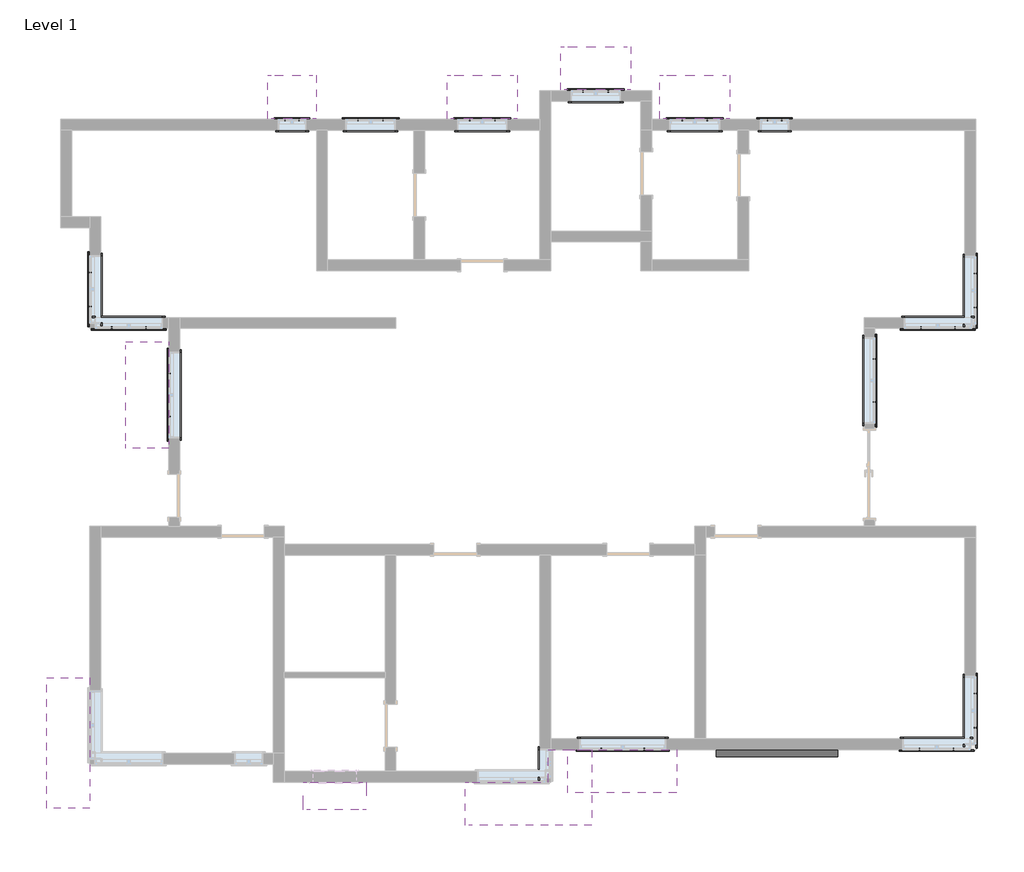
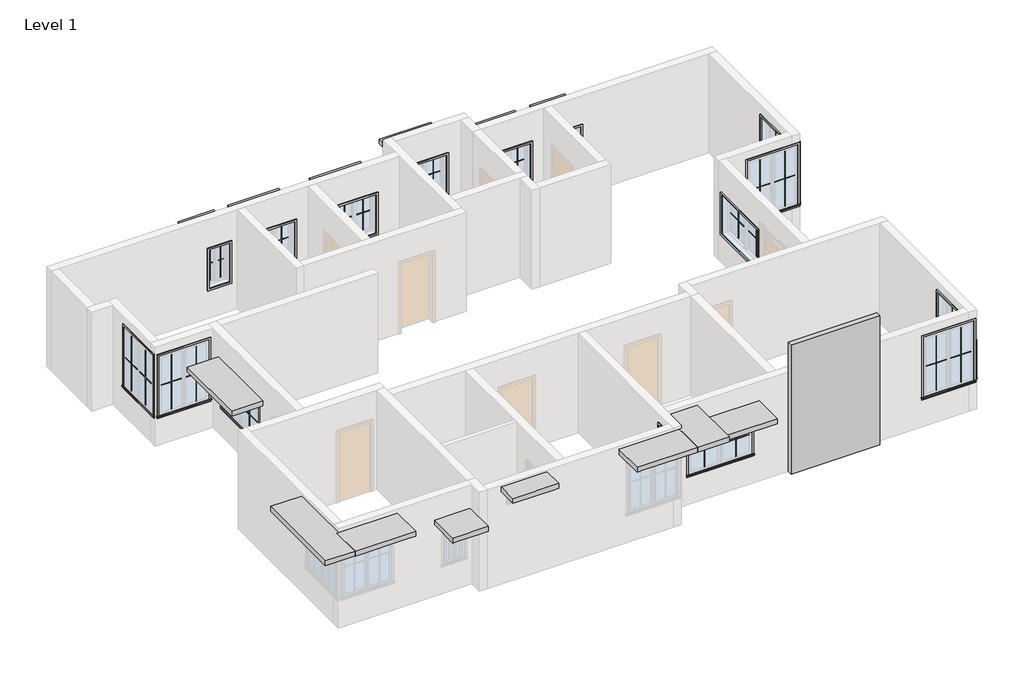
# One storey, part 3 of 3: 71 proxies.
"""IFC4 building model written with IfcOpenShell, lengths in millimetres."""

from ifc_helpers import new_model, si_unit, origin, place, context, project, spatial, transform, mapped, element, save
from components import generic_models_1_generic_models_1_0485f0a6, generic_models_13_generic_models_13_60817c59, generic_models_2_generic_models_2_5dfb3e49, generic_models_3_generic_models_3_1965cac1, generic_models_4_generic_models_4_668f170e, generic_models_5_generic_models_5_4455ebe8, generic_models_6_generic_models_6_772fa5ba, generic_models_7_generic_models_7_55042171, generic_models_8_generic_models_8_7ecb40ae, generic_models_9_generic_models_9_114c8f56, muntin_pattern_2x2_muntin_pattern_2x2_ddac5204, muntin_pattern_2x2_muntin_pattern_2x2_784a3213, muntin_pattern_2x2_muntin_pattern_2x2_dc2504c2, muntin_pattern_2x2_muntin_pattern_2x2_0aa094e9, muntin_pattern_2x2_muntin_pattern_2x2_63e5058f, muntin_pattern_2x2_muntin_pattern_2x2_529c3de1, muntin_pattern_2x2_muntin_pattern_2x2_bff912c5, muntin_pattern_2x2_muntin_pattern_2x2_c2194282, trim_window_exterior_flat_with_sill_35723329, trim_window_exterior_flat_with_sill_02d88a07, trim_window_exterior_flat_with_sill_245f2bb1, trim_window_exterior_flat_with_sill_e04b3088, trim_window_interior_flat_picture_frame_e16bff95, trim_window_interior_flat_picture_frame_03e64d7c, trim_window_interior_flat_picture_frame_2b4ba637, trim_window_interior_flat_picture_frame_2a7685fe, trim_window_interior_flat_picture_frame_6ac783dc

model = new_model("IFC4")

# Units and contexts
model_context = context("Model", 3, world=origin())
ifc_project = project(units=[si_unit("LENGTHUNIT", "METRE", prefix="MILLI")], contexts=[model_context])

# Site, building, storey
site = spatial("IfcSite", under=ifc_project)
building = spatial("IfcBuilding", under=site)
storey = spatial("IfcBuildingStorey", under=building, Name="Level 1", Elevation=0.0)

# Proxies
placement = place(None, origin())
generic_models_1_generic_models_1_shape = generic_models_1_generic_models_1_0485f0a6(model_context)
element("IfcBuildingElementProxy", 1, Name="Generic Models 1 : Generic Models 1", ObjectType="Generic Models 1 : Generic Models 1", at=placement, inside=storey, context=model_context, shape_type="MappedRepresentation", body=[
    mapped(generic_models_1_generic_models_1_shape, transform((0.0, 0.0, 0.0), x_axis=(1.0, 0.0, 0.0), y_axis=(0.0, 1.0, 0.0), z_axis=(0.0, 0.0, 1.0))),
])
generic_models_13_generic_models_13_shape = generic_models_13_generic_models_13_60817c59(model_context)
element("IfcBuildingElementProxy", 2, Name="Generic Models 13 : Generic Models 13", ObjectType="Generic Models 13 : Generic Models 13", at=placement, inside=storey, context=model_context, shape_type="MappedRepresentation", body=[
    mapped(generic_models_13_generic_models_13_shape, transform((0.0, 0.0, 0.0), x_axis=(1.0, 0.0, 0.0), y_axis=(0.0, 1.0, 0.0), z_axis=(0.0, 0.0, 1.0))),
])
generic_models_2_generic_models_2_shape = generic_models_2_generic_models_2_5dfb3e49(model_context)
element("IfcBuildingElementProxy", 3, Name="Generic Models 2 : Generic Models 2", ObjectType="Generic Models 2 : Generic Models 2", at=placement, inside=storey, context=model_context, shape_type="MappedRepresentation", body=[
    mapped(generic_models_2_generic_models_2_shape, transform((0.0, 0.0, 0.0), x_axis=(1.0, 0.0, 0.0), y_axis=(0.0, 1.0, 0.0), z_axis=(0.0, 0.0, 1.0))),
])
generic_models_3_generic_models_3_shape = generic_models_3_generic_models_3_1965cac1(model_context)
element("IfcBuildingElementProxy", 4, Name="Generic Models 3 : Generic Models 3", ObjectType="Generic Models 3 : Generic Models 3", at=placement, inside=storey, context=model_context, shape_type="MappedRepresentation", body=[
    mapped(generic_models_3_generic_models_3_shape, transform((-51.3527819, 0.0, 0.0272468), x_axis=(1.0, 0.0, 0.0), y_axis=(0.0, 1.0, 0.0), z_axis=(0.0, 0.0, 1.0))),
])
generic_models_4_generic_models_4_shape = generic_models_4_generic_models_4_668f170e(model_context)
element("IfcBuildingElementProxy", 5, Name="Generic Models 4 : Generic Models 4", ObjectType="Generic Models 4 : Generic Models 4", at=placement, inside=storey, context=model_context, shape_type="MappedRepresentation", body=[
    mapped(generic_models_4_generic_models_4_shape, transform((0.0, 0.0, 0.0), x_axis=(1.0, 0.0, 0.0), y_axis=(0.0, 1.0, 0.0), z_axis=(0.0, 0.0, 1.0))),
])
generic_models_5_generic_models_5_shape = generic_models_5_generic_models_5_4455ebe8(model_context)
element("IfcBuildingElementProxy", 6, Name="Generic Models 5 : Generic Models 5", ObjectType="Generic Models 5 : Generic Models 5", at=placement, inside=storey, context=model_context, shape_type="MappedRepresentation", body=[
    mapped(generic_models_5_generic_models_5_shape, transform((0.0, 0.0, 0.0), x_axis=(1.0, 0.0, 0.0), y_axis=(0.0, 1.0, 0.0), z_axis=(0.0, 0.0, 1.0))),
])
generic_models_6_generic_models_6_shape = generic_models_6_generic_models_6_772fa5ba(model_context)
element("IfcBuildingElementProxy", 7, Name="Generic Models 6 : Generic Models 6", ObjectType="Generic Models 6 : Generic Models 6", at=placement, inside=storey, context=model_context, shape_type="MappedRepresentation", body=[
    mapped(generic_models_6_generic_models_6_shape, transform((0.0, 0.0, 0.0), x_axis=(1.0, 0.0, 0.0), y_axis=(0.0, 1.0, 0.0), z_axis=(0.0, 0.0, 1.0))),
])
generic_models_7_generic_models_7_shape = generic_models_7_generic_models_7_55042171(model_context)
element("IfcBuildingElementProxy", 8, Name="Generic Models 7 : Generic Models 7", ObjectType="Generic Models 7 : Generic Models 7", at=placement, inside=storey, context=model_context, shape_type="MappedRepresentation", body=[
    mapped(generic_models_7_generic_models_7_shape, transform((0.0, 0.0, 0.0), x_axis=(1.0, 0.0, 0.0), y_axis=(0.0, 1.0, 0.0), z_axis=(0.0, 0.0, 1.0))),
])
generic_models_8_generic_models_8_shape = generic_models_8_generic_models_8_7ecb40ae(model_context)
element("IfcBuildingElementProxy", 9, Name="Generic Models 8 : Generic Models 8", ObjectType="Generic Models 8 : Generic Models 8", at=placement, inside=storey, context=model_context, shape_type="MappedRepresentation", body=[
    mapped(generic_models_8_generic_models_8_shape, transform((0.0, 0.0, 0.0), x_axis=(1.0, 0.0, 0.0), y_axis=(0.0, 1.0, 0.0), z_axis=(0.0, 0.0, 1.0))),
])
generic_models_9_generic_models_9_shape = generic_models_9_generic_models_9_114c8f56(model_context)
element("IfcBuildingElementProxy", 10, Name="Generic Models 9 : Generic Models 9", ObjectType="Generic Models 9 : Generic Models 9", at=placement, inside=storey, context=model_context, shape_type="MappedRepresentation", body=[
    mapped(generic_models_9_generic_models_9_shape, transform((0.0, 0.0, 0.0), x_axis=(1.0, 0.0, 0.0), y_axis=(0.0, 1.0, 0.0), z_axis=(0.0, 0.0, 1.0))),
])
muntin_pattern_2x2_muntin_pattern_2x2_shape = muntin_pattern_2x2_muntin_pattern_2x2_ddac5204(model_context)
element("IfcBuildingElementProxy", 11, Name="Muntin Pattern_2x2 : Muntin Pattern_2x2", ObjectType="Muntin Pattern_2x2 : Muntin Pattern_2x2", at=placement, inside=storey, context=model_context, shape_type="MappedRepresentation", body=[
    mapped(muntin_pattern_2x2_muntin_pattern_2x2_shape, transform((-27733.7270004, 19654.2006148, 984.25), x_axis=(1.0, 0.0, 0.0), y_axis=(0.0, 1.0, 0.0), z_axis=(0.0, 0.0, 1.0))),
])
element("IfcBuildingElementProxy", 12, Name="Muntin Pattern_2x2 : Muntin Pattern_2x2", ObjectType="Muntin Pattern_2x2 : Muntin Pattern_2x2", at=placement, inside=storey, context=model_context, shape_type="MappedRepresentation", body=[
    mapped(muntin_pattern_2x2_muntin_pattern_2x2_shape, transform((-37944.5270004, 19654.2006148, 984.25), x_axis=(1.0, 0.0, 0.0), y_axis=(0.0, 1.0, 0.0), z_axis=(0.0, 0.0, 1.0))),
])
muntin_pattern_2x2_muntin_pattern_2x2_2_shape = muntin_pattern_2x2_muntin_pattern_2x2_784a3213(model_context)
element("IfcBuildingElementProxy", 13, Name="Muntin Pattern_2x2 : Muntin Pattern_2x2", ObjectType="Muntin Pattern_2x2 : Muntin Pattern_2x2", at=placement, inside=storey, context=model_context, shape_type="MappedRepresentation", body=[
    mapped(muntin_pattern_2x2_muntin_pattern_2x2_2_shape, transform((-27432.1020004, 19654.2006148, 984.25), x_axis=(-1.0, 0.0, 0.0), y_axis=(0.0, -1.0, 0.0), z_axis=(0.0, 0.0, 1.0))),
])
element("IfcBuildingElementProxy", 14, Name="Muntin Pattern_2x2 : Muntin Pattern_2x2", ObjectType="Muntin Pattern_2x2 : Muntin Pattern_2x2", at=placement, inside=storey, context=model_context, shape_type="MappedRepresentation", body=[
    mapped(muntin_pattern_2x2_muntin_pattern_2x2_2_shape, transform((-37642.9020004, 19654.2006148, 984.25), x_axis=(-1.0, 0.0, 0.0), y_axis=(0.0, -1.0, 0.0), z_axis=(0.0, 0.0, 1.0))),
])
muntin_pattern_2x2_muntin_pattern_2x2_3_shape = muntin_pattern_2x2_muntin_pattern_2x2_dc2504c2(model_context)
element("IfcBuildingElementProxy", 15, Name="Muntin Pattern_2x2 : Muntin Pattern_2x2", ObjectType="Muntin Pattern_2x2 : Muntin Pattern_2x2", at=placement, inside=storey, context=model_context, shape_type="MappedRepresentation", body=[
    mapped(muntin_pattern_2x2_muntin_pattern_2x2_3_shape, transform((-30340.4020004, 6338.2506148, 984.25), x_axis=(-1.0, 0.0, 0.0), y_axis=(0.0, -1.0, 0.0), z_axis=(0.0, 0.0, 1.0))),
])
element("IfcBuildingElementProxy", 16, Name="Muntin Pattern_2x2 : Muntin Pattern_2x2", ObjectType="Muntin Pattern_2x2 : Muntin Pattern_2x2", at=placement, inside=storey, context=model_context, shape_type="MappedRepresentation", body=[
    mapped(muntin_pattern_2x2_muntin_pattern_2x2_3_shape, transform((-25471.5395004, 14594.8381148, 984.25), x_axis=(0.0, -1.0, 0.0), y_axis=(1.0, 0.0, 0.0), z_axis=(0.0, 0.0, 1.0))),
])
element("IfcBuildingElementProxy", 17, Name="Muntin Pattern_2x2 : Muntin Pattern_2x2", ObjectType="Muntin Pattern_2x2 : Muntin Pattern_2x2", at=placement, inside=storey, context=model_context, shape_type="MappedRepresentation", body=[
    mapped(muntin_pattern_2x2_muntin_pattern_2x2_3_shape, transform((-40387.6895004, 13378.8131148, 984.25), x_axis=(0.0, 1.0, 0.0), y_axis=(-1.0, 0.0, 0.0), z_axis=(0.0, 0.0, 1.0))),
])
muntin_pattern_2x2_muntin_pattern_2x2_4_shape = muntin_pattern_2x2_muntin_pattern_2x2_0aa094e9(model_context)
element("IfcBuildingElementProxy", 18, Name="Muntin Pattern_2x2 : Muntin Pattern_2x2", ObjectType="Muntin Pattern_2x2 : Muntin Pattern_2x2", at=placement, inside=storey, context=model_context, shape_type="MappedRepresentation", body=[
    mapped(muntin_pattern_2x2_muntin_pattern_2x2_4_shape, transform((-31251.6270004, 6338.2506148, 984.25), x_axis=(1.0, 0.0, 0.0), y_axis=(0.0, 1.0, 0.0), z_axis=(0.0, 0.0, 1.0))),
])
element("IfcBuildingElementProxy", 19, Name="Muntin Pattern_2x2 : Muntin Pattern_2x2", ObjectType="Muntin Pattern_2x2 : Muntin Pattern_2x2", at=placement, inside=storey, context=model_context, shape_type="MappedRepresentation", body=[
    mapped(muntin_pattern_2x2_muntin_pattern_2x2_4_shape, transform((-25471.5395004, 13683.6131148, 984.25), x_axis=(0.0, 1.0, 0.0), y_axis=(-1.0, 0.0, 0.0), z_axis=(0.0, 0.0, 1.0))),
])
element("IfcBuildingElementProxy", 20, Name="Muntin Pattern_2x2 : Muntin Pattern_2x2", ObjectType="Muntin Pattern_2x2 : Muntin Pattern_2x2", at=placement, inside=storey, context=model_context, shape_type="MappedRepresentation", body=[
    mapped(muntin_pattern_2x2_muntin_pattern_2x2_4_shape, transform((-40387.6895004, 14290.0381148, 984.25), x_axis=(0.0, -1.0, 0.0), y_axis=(1.0, 0.0, 0.0), z_axis=(0.0, 0.0, 1.0))),
])
muntin_pattern_2x2_muntin_pattern_2x2_5_shape = muntin_pattern_2x2_muntin_pattern_2x2_63e5058f(model_context)
element("IfcBuildingElementProxy", 21, Name="Muntin Pattern_2x2 : Muntin Pattern_2x2", ObjectType="Muntin Pattern_2x2 : Muntin Pattern_2x2", at=placement, inside=storey, context=model_context, shape_type="MappedRepresentation", body=[
    mapped(muntin_pattern_2x2_muntin_pattern_2x2_5_shape, transform((-36395.1270004, 19654.2006148, 984.25), x_axis=(1.0, 0.0, 0.0), y_axis=(0.0, 1.0, 0.0), z_axis=(0.0, 0.0, 1.0))),
])
element("IfcBuildingElementProxy", 22, Name="Muntin Pattern_2x2 : Muntin Pattern_2x2", ObjectType="Muntin Pattern_2x2 : Muntin Pattern_2x2", at=placement, inside=storey, context=model_context, shape_type="MappedRepresentation", body=[
    mapped(muntin_pattern_2x2_muntin_pattern_2x2_5_shape, transform((-34032.9270004, 19654.2006148, 984.25), x_axis=(1.0, 0.0, 0.0), y_axis=(0.0, 1.0, 0.0), z_axis=(0.0, 0.0, 1.0))),
])
element("IfcBuildingElementProxy", 23, Name="Muntin Pattern_2x2 : Muntin Pattern_2x2", ObjectType="Muntin Pattern_2x2 : Muntin Pattern_2x2", at=placement, inside=storey, context=model_context, shape_type="MappedRepresentation", body=[
    mapped(muntin_pattern_2x2_muntin_pattern_2x2_5_shape, transform((-31632.6270004, 20263.8006148, 984.25), x_axis=(1.0, 0.0, 0.0), y_axis=(0.0, 1.0, 0.0), z_axis=(0.0, 0.0, 1.0))),
])
element("IfcBuildingElementProxy", 24, Name="Muntin Pattern_2x2 : Muntin Pattern_2x2", ObjectType="Muntin Pattern_2x2 : Muntin Pattern_2x2", at=placement, inside=storey, context=model_context, shape_type="MappedRepresentation", body=[
    mapped(muntin_pattern_2x2_muntin_pattern_2x2_5_shape, transform((-29537.1270004, 19654.2006148, 984.25), x_axis=(1.0, 0.0, 0.0), y_axis=(0.0, 1.0, 0.0), z_axis=(0.0, 0.0, 1.0))),
])
muntin_pattern_2x2_muntin_pattern_2x2_6_shape = muntin_pattern_2x2_muntin_pattern_2x2_529c3de1(model_context)
element("IfcBuildingElementProxy", 25, Name="Muntin Pattern_2x2 : Muntin Pattern_2x2", ObjectType="Muntin Pattern_2x2 : Muntin Pattern_2x2", at=placement, inside=storey, context=model_context, shape_type="MappedRepresentation", body=[
    mapped(muntin_pattern_2x2_muntin_pattern_2x2_6_shape, transform((-35864.9020004, 19654.2006148, 984.25), x_axis=(-1.0, 0.0, 0.0), y_axis=(0.0, -1.0, 0.0), z_axis=(0.0, 0.0, 1.0))),
])
element("IfcBuildingElementProxy", 26, Name="Muntin Pattern_2x2 : Muntin Pattern_2x2", ObjectType="Muntin Pattern_2x2 : Muntin Pattern_2x2", at=placement, inside=storey, context=model_context, shape_type="MappedRepresentation", body=[
    mapped(muntin_pattern_2x2_muntin_pattern_2x2_6_shape, transform((-33502.7020004, 19654.2006148, 984.25), x_axis=(-1.0, 0.0, 0.0), y_axis=(0.0, -1.0, 0.0), z_axis=(0.0, 0.0, 1.0))),
])
element("IfcBuildingElementProxy", 27, Name="Muntin Pattern_2x2 : Muntin Pattern_2x2", ObjectType="Muntin Pattern_2x2 : Muntin Pattern_2x2", at=placement, inside=storey, context=model_context, shape_type="MappedRepresentation", body=[
    mapped(muntin_pattern_2x2_muntin_pattern_2x2_6_shape, transform((-31102.4020004, 20263.8006148, 984.25), x_axis=(-1.0, 0.0, 0.0), y_axis=(0.0, -1.0, 0.0), z_axis=(0.0, 0.0, 1.0))),
])
element("IfcBuildingElementProxy", 28, Name="Muntin Pattern_2x2 : Muntin Pattern_2x2", ObjectType="Muntin Pattern_2x2 : Muntin Pattern_2x2", at=placement, inside=storey, context=model_context, shape_type="MappedRepresentation", body=[
    mapped(muntin_pattern_2x2_muntin_pattern_2x2_6_shape, transform((-29006.9020004, 19654.2006148, 984.25), x_axis=(-1.0, 0.0, 0.0), y_axis=(0.0, -1.0, 0.0), z_axis=(0.0, 0.0, 1.0))),
])
muntin_pattern_2x2_muntin_pattern_2x2_7_shape = muntin_pattern_2x2_muntin_pattern_2x2_bff912c5(model_context)
element("IfcBuildingElementProxy", 29, Name="Muntin Pattern_2x2 : Muntin Pattern_2x2", ObjectType="Muntin Pattern_2x2 : Muntin Pattern_2x2", at=placement, inside=storey, context=model_context, shape_type="MappedRepresentation", body=[
    mapped(muntin_pattern_2x2_muntin_pattern_2x2_7_shape, transform((-23793.5520004, 6338.2506148, 984.25), x_axis=(-1.0, 0.0, 0.0), y_axis=(0.0, -1.0, 0.0), z_axis=(0.0, 0.0, 1.0))),
])
element("IfcBuildingElementProxy", 30, Name="Muntin Pattern_2x2 : Muntin Pattern_2x2", ObjectType="Muntin Pattern_2x2 : Muntin Pattern_2x2", at=placement, inside=storey, context=model_context, shape_type="MappedRepresentation", body=[
    mapped(muntin_pattern_2x2_muntin_pattern_2x2_7_shape, transform((-23337.9395004, 7514.5881148, 984.25), x_axis=(0.0, -1.0, 0.0), y_axis=(1.0, 0.0, 0.0), z_axis=(0.0, 0.0, 1.0))),
])
element("IfcBuildingElementProxy", 31, Name="Muntin Pattern_2x2 : Muntin Pattern_2x2", ObjectType="Muntin Pattern_2x2 : Muntin Pattern_2x2", at=placement, inside=storey, context=model_context, shape_type="MappedRepresentation", body=[
    mapped(muntin_pattern_2x2_muntin_pattern_2x2_7_shape, transform((-23768.1520004, 15253.6506148, 984.25), x_axis=(-1.0, 0.0, 0.0), y_axis=(0.0, -1.0, 0.0), z_axis=(0.0, 0.0, 1.0))),
])
element("IfcBuildingElementProxy", 32, Name="Muntin Pattern_2x2 : Muntin Pattern_2x2", ObjectType="Muntin Pattern_2x2 : Muntin Pattern_2x2", at=placement, inside=storey, context=model_context, shape_type="MappedRepresentation", body=[
    mapped(muntin_pattern_2x2_muntin_pattern_2x2_7_shape, transform((-23337.9395004, 16404.5881148, 984.25), x_axis=(0.0, -1.0, 0.0), y_axis=(1.0, 0.0, 0.0), z_axis=(0.0, 0.0, 1.0))),
])
element("IfcBuildingElementProxy", 33, Name="Muntin Pattern_2x2 : Muntin Pattern_2x2", ObjectType="Muntin Pattern_2x2 : Muntin Pattern_2x2", at=placement, inside=storey, context=model_context, shape_type="MappedRepresentation", body=[
    mapped(muntin_pattern_2x2_muntin_pattern_2x2_7_shape, transform((-40887.7520004, 15253.6506148, 984.25), x_axis=(-1.0, 0.0, 0.0), y_axis=(0.0, -1.0, 0.0), z_axis=(0.0, 0.0, 1.0))),
])
element("IfcBuildingElementProxy", 34, Name="Muntin Pattern_2x2 : Muntin Pattern_2x2", ObjectType="Muntin Pattern_2x2 : Muntin Pattern_2x2", at=placement, inside=storey, context=model_context, shape_type="MappedRepresentation", body=[
    mapped(muntin_pattern_2x2_muntin_pattern_2x2_7_shape, transform((-42064.0895004, 15709.2631148, 984.25), x_axis=(0.0, 1.0, 0.0), y_axis=(-1.0, 0.0, 0.0), z_axis=(0.0, 0.0, 1.0))),
])
muntin_pattern_2x2_muntin_pattern_2x2_8_shape = muntin_pattern_2x2_muntin_pattern_2x2_c2194282(model_context)
element("IfcBuildingElementProxy", 35, Name="Muntin Pattern_2x2 : Muntin Pattern_2x2", ObjectType="Muntin Pattern_2x2 : Muntin Pattern_2x2", at=placement, inside=storey, context=model_context, shape_type="MappedRepresentation", body=[
    mapped(muntin_pattern_2x2_muntin_pattern_2x2_8_shape, transform((-24514.2770004, 6338.2506148, 984.25), x_axis=(1.0, 0.0, 0.0), y_axis=(0.0, 1.0, 0.0), z_axis=(0.0, 0.0, 1.0))),
])
element("IfcBuildingElementProxy", 36, Name="Muntin Pattern_2x2 : Muntin Pattern_2x2", ObjectType="Muntin Pattern_2x2 : Muntin Pattern_2x2", at=placement, inside=storey, context=model_context, shape_type="MappedRepresentation", body=[
    mapped(muntin_pattern_2x2_muntin_pattern_2x2_8_shape, transform((-23337.9395004, 6793.8631148, 984.25), x_axis=(0.0, 1.0, 0.0), y_axis=(-1.0, 0.0, 0.0), z_axis=(0.0, 0.0, 1.0))),
])
element("IfcBuildingElementProxy", 37, Name="Muntin Pattern_2x2 : Muntin Pattern_2x2", ObjectType="Muntin Pattern_2x2 : Muntin Pattern_2x2", at=placement, inside=storey, context=model_context, shape_type="MappedRepresentation", body=[
    mapped(muntin_pattern_2x2_muntin_pattern_2x2_8_shape, transform((-24488.8770004, 15253.6506148, 984.25), x_axis=(1.0, 0.0, 0.0), y_axis=(0.0, 1.0, 0.0), z_axis=(0.0, 0.0, 1.0))),
])
element("IfcBuildingElementProxy", 38, Name="Muntin Pattern_2x2 : Muntin Pattern_2x2", ObjectType="Muntin Pattern_2x2 : Muntin Pattern_2x2", at=placement, inside=storey, context=model_context, shape_type="MappedRepresentation", body=[
    mapped(muntin_pattern_2x2_muntin_pattern_2x2_8_shape, transform((-23337.9395004, 15683.8631148, 984.25), x_axis=(0.0, 1.0, 0.0), y_axis=(-1.0, 0.0, 0.0), z_axis=(0.0, 0.0, 1.0))),
])
element("IfcBuildingElementProxy", 39, Name="Muntin Pattern_2x2 : Muntin Pattern_2x2", ObjectType="Muntin Pattern_2x2 : Muntin Pattern_2x2", at=placement, inside=storey, context=model_context, shape_type="MappedRepresentation", body=[
    mapped(muntin_pattern_2x2_muntin_pattern_2x2_8_shape, transform((-41608.4770004, 15253.6506148, 984.25), x_axis=(1.0, 0.0, 0.0), y_axis=(0.0, 1.0, 0.0), z_axis=(0.0, 0.0, 1.0))),
])
element("IfcBuildingElementProxy", 40, Name="Muntin Pattern_2x2 : Muntin Pattern_2x2", ObjectType="Muntin Pattern_2x2 : Muntin Pattern_2x2", at=placement, inside=storey, context=model_context, shape_type="MappedRepresentation", body=[
    mapped(muntin_pattern_2x2_muntin_pattern_2x2_8_shape, transform((-42064.0895004, 16429.9881148, 984.25), x_axis=(0.0, -1.0, 0.0), y_axis=(1.0, 0.0, 0.0), z_axis=(0.0, 0.0, 1.0))),
])
trim_window_exterior_flat_with_sill_shape = trim_window_exterior_flat_with_sill_35723329(model_context)
element("IfcBuildingElementProxy", 41, Name="Trim-Window-Exterior-Flat : with Sill", ObjectType="Trim-Window-Exterior-Flat : with Sill", at=placement, inside=storey, context=model_context, shape_type="MappedRepresentation", body=[
    mapped(trim_window_exterior_flat_with_sill_shape, transform((-27582.9145004, 19663.7256148, 2133.6), x_axis=(-1.0, 0.0, 0.0), y_axis=(0.0, 0.0, 1.0), z_axis=(0.0, 1.0, 0.0))),
])
element("IfcBuildingElementProxy", 42, Name="Trim-Window-Exterior-Flat : with Sill", ObjectType="Trim-Window-Exterior-Flat : with Sill", at=placement, inside=storey, context=model_context, shape_type="MappedRepresentation", body=[
    mapped(trim_window_exterior_flat_with_sill_shape, transform((-37793.7145004, 19663.7256148, 2133.6), x_axis=(-1.0, 0.0, 0.0), y_axis=(0.0, 0.0, 1.0), z_axis=(0.0, 1.0, 0.0))),
])
trim_window_exterior_flat_with_sill_2_shape = trim_window_exterior_flat_with_sill_02d88a07(model_context)
element("IfcBuildingElementProxy", 43, Name="Trim-Window-Exterior-Flat : with Sill", ObjectType="Trim-Window-Exterior-Flat : with Sill", at=placement, inside=storey, context=model_context, shape_type="MappedRepresentation", body=[
    mapped(trim_window_exterior_flat_with_sill_2_shape, transform((-30796.0145004, 6328.7256148, 2133.6), x_axis=(1.0, 0.0, 0.0), y_axis=(0.0, 0.0, 1.0), z_axis=(0.0, -1.0, 0.0))),
])
element("IfcBuildingElementProxy", 44, Name="Trim-Window-Exterior-Flat : with Sill", ObjectType="Trim-Window-Exterior-Flat : with Sill", at=placement, inside=storey, context=model_context, shape_type="MappedRepresentation", body=[
    mapped(trim_window_exterior_flat_with_sill_2_shape, transform((-25462.0145004, 14139.2256148, 2133.6), x_axis=(0.0, 1.0, 0.0), y_axis=(0.0, 0.0, 1.0), z_axis=(1.0, 0.0, 0.0))),
])
element("IfcBuildingElementProxy", 45, Name="Trim-Window-Exterior-Flat : with Sill", ObjectType="Trim-Window-Exterior-Flat : with Sill", at=placement, inside=storey, context=model_context, shape_type="MappedRepresentation", body=[
    mapped(trim_window_exterior_flat_with_sill_2_shape, transform((-40397.2145004, 13834.4256148, 2133.6), x_axis=(0.0, -1.0, 0.0), y_axis=(0.0, 0.0, 1.0), z_axis=(-1.0, 0.0, 0.0))),
])
trim_window_exterior_flat_with_sill_3_shape = trim_window_exterior_flat_with_sill_245f2bb1(model_context)
element("IfcBuildingElementProxy", 46, Name="Trim-Window-Exterior-Flat : with Sill", ObjectType="Trim-Window-Exterior-Flat : with Sill", at=placement, inside=storey, context=model_context, shape_type="MappedRepresentation", body=[
    mapped(trim_window_exterior_flat_with_sill_3_shape, transform((-36130.0145004, 19663.7256148, 2133.6), x_axis=(-1.0, 0.0, 0.0), y_axis=(0.0, 0.0, 1.0), z_axis=(0.0, 1.0, 0.0))),
])
element("IfcBuildingElementProxy", 47, Name="Trim-Window-Exterior-Flat : with Sill", ObjectType="Trim-Window-Exterior-Flat : with Sill", at=placement, inside=storey, context=model_context, shape_type="MappedRepresentation", body=[
    mapped(trim_window_exterior_flat_with_sill_3_shape, transform((-33767.8145004, 19663.7256148, 2133.6), x_axis=(-1.0, 0.0, 0.0), y_axis=(0.0, 0.0, 1.0), z_axis=(0.0, 1.0, 0.0))),
])
element("IfcBuildingElementProxy", 48, Name="Trim-Window-Exterior-Flat : with Sill", ObjectType="Trim-Window-Exterior-Flat : with Sill", at=placement, inside=storey, context=model_context, shape_type="MappedRepresentation", body=[
    mapped(trim_window_exterior_flat_with_sill_3_shape, transform((-31367.5145004, 20273.3256148, 2133.6), x_axis=(-1.0, 0.0, 0.0), y_axis=(0.0, 0.0, 1.0), z_axis=(0.0, 1.0, 0.0))),
])
element("IfcBuildingElementProxy", 49, Name="Trim-Window-Exterior-Flat : with Sill", ObjectType="Trim-Window-Exterior-Flat : with Sill", at=placement, inside=storey, context=model_context, shape_type="MappedRepresentation", body=[
    mapped(trim_window_exterior_flat_with_sill_3_shape, transform((-29272.0145004, 19663.7256148, 2133.6), x_axis=(-1.0, 0.0, 0.0), y_axis=(0.0, 0.0, 1.0), z_axis=(0.0, 1.0, 0.0))),
])
trim_window_exterior_flat_with_sill_4_shape = trim_window_exterior_flat_with_sill_e04b3088(model_context)
element("IfcBuildingElementProxy", 50, Name="Trim-Window-Exterior-Flat : with Sill", ObjectType="Trim-Window-Exterior-Flat : with Sill", at=placement, inside=storey, context=model_context, shape_type="MappedRepresentation", body=[
    mapped(trim_window_exterior_flat_with_sill_4_shape, transform((-24153.9145004, 6328.7256148, 2743.2), x_axis=(1.0, 0.0, 0.0), y_axis=(0.0, 0.0, 1.0), z_axis=(0.0, -1.0, 0.0))),
])
element("IfcBuildingElementProxy", 51, Name="Trim-Window-Exterior-Flat : with Sill", ObjectType="Trim-Window-Exterior-Flat : with Sill", at=placement, inside=storey, context=model_context, shape_type="MappedRepresentation", body=[
    mapped(trim_window_exterior_flat_with_sill_4_shape, transform((-23328.4145004, 7154.2256148, 2743.2), x_axis=(0.0, 1.0, 0.0), y_axis=(0.0, 0.0, 1.0), z_axis=(1.0, 0.0, 0.0))),
])
element("IfcBuildingElementProxy", 52, Name="Trim-Window-Exterior-Flat : with Sill", ObjectType="Trim-Window-Exterior-Flat : with Sill", at=placement, inside=storey, context=model_context, shape_type="MappedRepresentation", body=[
    mapped(trim_window_exterior_flat_with_sill_4_shape, transform((-24128.5145004, 15244.1256148, 2743.2), x_axis=(1.0, 0.0, 0.0), y_axis=(0.0, 0.0, 1.0), z_axis=(0.0, -1.0, 0.0))),
])
element("IfcBuildingElementProxy", 53, Name="Trim-Window-Exterior-Flat : with Sill", ObjectType="Trim-Window-Exterior-Flat : with Sill", at=placement, inside=storey, context=model_context, shape_type="MappedRepresentation", body=[
    mapped(trim_window_exterior_flat_with_sill_4_shape, transform((-23328.4145004, 16044.2256148, 2743.2), x_axis=(0.0, 1.0, 0.0), y_axis=(0.0, 0.0, 1.0), z_axis=(1.0, 0.0, 0.0))),
])
element("IfcBuildingElementProxy", 54, Name="Trim-Window-Exterior-Flat : with Sill", ObjectType="Trim-Window-Exterior-Flat : with Sill", at=placement, inside=storey, context=model_context, shape_type="MappedRepresentation", body=[
    mapped(trim_window_exterior_flat_with_sill_4_shape, transform((-41248.1145004, 15244.1256148, 2743.2), x_axis=(1.0, 0.0, 0.0), y_axis=(0.0, 0.0, 1.0), z_axis=(0.0, -1.0, 0.0))),
])
element("IfcBuildingElementProxy", 55, Name="Trim-Window-Exterior-Flat : with Sill", ObjectType="Trim-Window-Exterior-Flat : with Sill", at=placement, inside=storey, context=model_context, shape_type="MappedRepresentation", body=[
    mapped(trim_window_exterior_flat_with_sill_4_shape, transform((-42073.6145004, 16069.6256148, 2743.2), x_axis=(0.0, -1.0, 0.0), y_axis=(0.0, 0.0, 1.0), z_axis=(-1.0, 0.0, 0.0))),
])
trim_window_interior_flat_picture_frame_shape = trim_window_interior_flat_picture_frame_e16bff95(model_context)
element("IfcBuildingElementProxy", 56, Name="Trim-Window-Interior-Flat : Picture Frame", ObjectType="Trim-Window-Interior-Flat : Picture Frame", at=placement, inside=storey, context=model_context, shape_type="MappedRepresentation", body=[
    mapped(trim_window_interior_flat_picture_frame_shape, transform((-27582.9145004, 19435.1256148, 2133.6), x_axis=(1.0, 0.0, 0.0), y_axis=(0.0, 0.0, 1.0), z_axis=(0.0, -1.0, 0.0))),
])
element("IfcBuildingElementProxy", 57, Name="Trim-Window-Interior-Flat : Picture Frame", ObjectType="Trim-Window-Interior-Flat : Picture Frame", at=placement, inside=storey, context=model_context, shape_type="MappedRepresentation", body=[
    mapped(trim_window_interior_flat_picture_frame_shape, transform((-37793.7145004, 19435.1256148, 2133.6), x_axis=(1.0, 0.0, 0.0), y_axis=(0.0, 0.0, 1.0), z_axis=(0.0, -1.0, 0.0))),
])
trim_window_interior_flat_picture_frame_2_shape = trim_window_interior_flat_picture_frame_03e64d7c(model_context)
element("IfcBuildingElementProxy", 58, Name="Trim-Window-Interior-Flat : Picture Frame", ObjectType="Trim-Window-Interior-Flat : Picture Frame", at=placement, inside=storey, context=model_context, shape_type="MappedRepresentation", body=[
    mapped(trim_window_interior_flat_picture_frame_2_shape, transform((-30796.0145004, 6557.3256148, 2133.6), x_axis=(-1.0, 0.0, 0.0), y_axis=(0.0, 0.0, 1.0), z_axis=(0.0, 1.0, 0.0))),
])
element("IfcBuildingElementProxy", 59, Name="Trim-Window-Interior-Flat : Picture Frame", ObjectType="Trim-Window-Interior-Flat : Picture Frame", at=placement, inside=storey, context=model_context, shape_type="MappedRepresentation", body=[
    mapped(trim_window_interior_flat_picture_frame_2_shape, transform((-25690.6145004, 14139.2256148, 2133.6), x_axis=(0.0, -1.0, 0.0), y_axis=(0.0, 0.0, 1.0), z_axis=(-1.0, 0.0, 0.0))),
])
element("IfcBuildingElementProxy", 60, Name="Trim-Window-Interior-Flat : Picture Frame", ObjectType="Trim-Window-Interior-Flat : Picture Frame", at=placement, inside=storey, context=model_context, shape_type="MappedRepresentation", body=[
    mapped(trim_window_interior_flat_picture_frame_2_shape, transform((-40168.6145004, 13834.4256148, 2133.6), x_axis=(0.0, 1.0, 0.0), y_axis=(0.0, 0.0, 1.0), z_axis=(1.0, 0.0, 0.0))),
])
trim_window_interior_flat_picture_frame_3_shape = trim_window_interior_flat_picture_frame_2b4ba637(model_context)
element("IfcBuildingElementProxy", 61, Name="Trim-Window-Interior-Flat : Picture Frame", ObjectType="Trim-Window-Interior-Flat : Picture Frame", at=placement, inside=storey, context=model_context, shape_type="MappedRepresentation", body=[
    mapped(trim_window_interior_flat_picture_frame_3_shape, transform((-36130.0145004, 19435.1256148, 2133.6), x_axis=(1.0, 0.0, 0.0), y_axis=(0.0, 0.0, 1.0), z_axis=(0.0, -1.0, 0.0))),
])
element("IfcBuildingElementProxy", 62, Name="Trim-Window-Interior-Flat : Picture Frame", ObjectType="Trim-Window-Interior-Flat : Picture Frame", at=placement, inside=storey, context=model_context, shape_type="MappedRepresentation", body=[
    mapped(trim_window_interior_flat_picture_frame_3_shape, transform((-33767.8145004, 19435.1256148, 2133.6), x_axis=(1.0, 0.0, 0.0), y_axis=(0.0, 0.0, 1.0), z_axis=(0.0, -1.0, 0.0))),
])
element("IfcBuildingElementProxy", 63, Name="Trim-Window-Interior-Flat : Picture Frame", ObjectType="Trim-Window-Interior-Flat : Picture Frame", at=placement, inside=storey, context=model_context, shape_type="MappedRepresentation", body=[
    mapped(trim_window_interior_flat_picture_frame_3_shape, transform((-31367.5145004, 20044.7256148, 2133.6), x_axis=(1.0, 0.0, 0.0), y_axis=(0.0, 0.0, 1.0), z_axis=(0.0, -1.0, 0.0))),
])
element("IfcBuildingElementProxy", 64, Name="Trim-Window-Interior-Flat : Picture Frame", ObjectType="Trim-Window-Interior-Flat : Picture Frame", at=placement, inside=storey, context=model_context, shape_type="MappedRepresentation", body=[
    mapped(trim_window_interior_flat_picture_frame_3_shape, transform((-29272.0145004, 19435.1256148, 2133.6), x_axis=(1.0, 0.0, 0.0), y_axis=(0.0, 0.0, 1.0), z_axis=(0.0, -1.0, 0.0))),
])
trim_window_interior_flat_picture_frame_4_shape = trim_window_interior_flat_picture_frame_2a7685fe(model_context)
element("IfcBuildingElementProxy", 65, Name="Trim-Window-Interior-Flat : Picture Frame", ObjectType="Trim-Window-Interior-Flat : Picture Frame", at=placement, inside=storey, context=model_context, shape_type="MappedRepresentation", body=[
    mapped(trim_window_interior_flat_picture_frame_4_shape, transform((-24153.9145004, 6557.3256148, 2743.2), x_axis=(-1.0, 0.0, 0.0), y_axis=(0.0, 0.0, 1.0), z_axis=(0.0, 1.0, 0.0))),
])
element("IfcBuildingElementProxy", 66, Name="Trim-Window-Interior-Flat : Picture Frame", ObjectType="Trim-Window-Interior-Flat : Picture Frame", at=placement, inside=storey, context=model_context, shape_type="MappedRepresentation", body=[
    mapped(trim_window_interior_flat_picture_frame_4_shape, transform((-23557.0145004, 7154.2256148, 2743.2), x_axis=(0.0, -1.0, 0.0), y_axis=(0.0, 0.0, 1.0), z_axis=(-1.0, 0.0, 0.0))),
])
element("IfcBuildingElementProxy", 67, Name="Trim-Window-Interior-Flat : Picture Frame", ObjectType="Trim-Window-Interior-Flat : Picture Frame", at=placement, inside=storey, context=model_context, shape_type="MappedRepresentation", body=[
    mapped(trim_window_interior_flat_picture_frame_4_shape, transform((-24128.5145004, 15472.7256148, 2743.2), x_axis=(-1.0, 0.0, 0.0), y_axis=(0.0, 0.0, 1.0), z_axis=(0.0, 1.0, 0.0))),
])
element("IfcBuildingElementProxy", 68, Name="Trim-Window-Interior-Flat : Picture Frame", ObjectType="Trim-Window-Interior-Flat : Picture Frame", at=placement, inside=storey, context=model_context, shape_type="MappedRepresentation", body=[
    mapped(trim_window_interior_flat_picture_frame_4_shape, transform((-23557.0145004, 16044.2256148, 2743.2), x_axis=(0.0, -1.0, 0.0), y_axis=(0.0, 0.0, 1.0), z_axis=(-1.0, 0.0, 0.0))),
])
element("IfcBuildingElementProxy", 69, Name="Trim-Window-Interior-Flat : Picture Frame", ObjectType="Trim-Window-Interior-Flat : Picture Frame", at=placement, inside=storey, context=model_context, shape_type="MappedRepresentation", body=[
    mapped(trim_window_interior_flat_picture_frame_4_shape, transform((-41248.1145004, 15472.7256148, 2743.2), x_axis=(-1.0, 0.0, 0.0), y_axis=(0.0, 0.0, 1.0), z_axis=(0.0, 1.0, 0.0))),
])
element("IfcBuildingElementProxy", 70, Name="Trim-Window-Interior-Flat : Picture Frame", ObjectType="Trim-Window-Interior-Flat : Picture Frame", at=placement, inside=storey, context=model_context, shape_type="MappedRepresentation", body=[
    mapped(trim_window_interior_flat_picture_frame_4_shape, transform((-41845.0145004, 16069.6256148, 2743.2), x_axis=(0.0, 1.0, 0.0), y_axis=(0.0, 0.0, 1.0), z_axis=(1.0, 0.0, 0.0))),
])
trim_window_interior_flat_picture_frame_5_shape = trim_window_interior_flat_picture_frame_6ac783dc(model_context)
element("IfcBuildingElementProxy", 71, Name="Trim-Window-Interior-Flat : Picture Frame", ObjectType="Trim-Window-Interior-Flat : Picture Frame", at=placement, inside=storey, context=model_context, shape_type="MappedRepresentation", body=[
    mapped(trim_window_interior_flat_picture_frame_5_shape, transform((-32548.6145004, 6036.5472085, 2743.2), x_axis=(0.0, -1.0, 0.0), y_axis=(0.0, 0.0, 1.0), z_axis=(-1.0, 0.0, 0.0))),
])

save(model, "model.ifc")

# Revit data of these elements
# Type "Muntin Pattern_2x2 : Muntin Pattern_2x2"
#   Width [instance default] = 4' - 0"
#   Thickness = 0' - 0 1/2"
#   Height [instance default] = 4' - 0"
#   Distance = 0' - 0 3/4"
#   Interior Material [instance default] = none
#   Exterior Material [instance default] = none
#   Default Elevation = 0
# Type "Trim-Window-Exterior-Flat : with Sill"
#   Trim Width = 0' - 2 1/4"
#   Trim Thickness_Picture Frame = 0' - 1 1/4"
#   Trim Thickness_with Sill = 0' - 0 3/4"
#   Sill Thickness = 0' - 1 1/4"
#   Opening Width [instance default] = 2' - 0"
#   Opening Height [instance default] = 3' - 0"
#   Default Elevation = 4' - 0"
#   Sill = yes
#   Picture Frame = no
#   Trim Material [instance default] = none
# Type "Trim-Window-Interior-Flat : Picture Frame"
#   Trim Thickness_Picture Frame = 0' - 1 1/4"
#   Trim Width = 0' - 2 1/4"
#   Trim Thickness_with Sill = 0' - 0 3/4"
#   Sill Thickness = 0' - 1 1/4"
#   Opening Width [instance default] = 2' - 0"
#   Opening Height [instance default] = 3' - 0"
#   Default Elevation = 4' - 0"
#   Sill = no
#   Picture Frame = yes
#   Trim Material [instance default] = none
# Element 1 (IfcBuildingElementProxy, "Generic Models 1 : Generic Models 1")
#   Phase Created = New Construction
# Element 2 (IfcBuildingElementProxy, "Generic Models 13 : Generic Models 13")
#   Phase Created = New Construction
# Element 3 (IfcBuildingElementProxy, "Generic Models 2 : Generic Models 2")
#   Phase Created = New Construction
# Element 4 (IfcBuildingElementProxy, "Generic Models 3 : Generic Models 3")
#   Phase Created = New Construction
# Element 5 (IfcBuildingElementProxy, "Generic Models 4 : Generic Models 4")
#   Phase Created = New Construction
# Element 6 (IfcBuildingElementProxy, "Generic Models 5 : Generic Models 5")
#   Phase Created = New Construction
# Element 7 (IfcBuildingElementProxy, "Generic Models 6 : Generic Models 6")
#   Phase Created = New Construction
# Element 8 (IfcBuildingElementProxy, "Generic Models 7 : Generic Models 7")
#   Phase Created = New Construction
# Element 9 (IfcBuildingElementProxy, "Generic Models 8 : Generic Models 8")
#   Phase Created = New Construction
# Element 10 (IfcBuildingElementProxy, "Generic Models 9 : Generic Models 9")
#   Phase Created = New Construction
# Elements 11, 12, 13, 14 (IfcBuildingElementProxy, "Muntin Pattern_2x2 : Muntin Pattern_2x2")
#   Width = 0' - 6 5/8"
#   Height = 3' - 6 1/2"
#   Interior Material = Wood - Stained
#   Exterior Material = Clad - White
#   Phase Created = New Construction
#   Materials on its faces: "Clad - White", "Wood - Stained"
# Elements 15, 16, 17, 18, 19, 20 (IfcBuildingElementProxy, "Muntin Pattern_2x2 : Muntin Pattern_2x2")
#   Width = 2' - 6 5/8"
#   Height = 3' - 6 1/2"
#   Interior Material = Wood - Stained
#   Exterior Material = Clad - White
#   Phase Created = New Construction
#   Materials on its faces: "Clad - White", "Wood - Stained"
# Elements 21, 22, 23, 24, 25, 26, 27, 28 (IfcBuildingElementProxy, "Muntin Pattern_2x2 : Muntin Pattern_2x2")
#   Width = 1' - 3 5/8"
#   Height = 3' - 6 1/2"
#   Interior Material = Wood - Stained
#   Exterior Material = Clad - White
#   Phase Created = New Construction
#   Materials on its faces: "Clad - White", "Wood - Stained"
# Elements 29, 30, 31, 32, 33, 34, 35, 36, 37, 38, 39, 40 (IfcBuildingElementProxy, "Muntin Pattern_2x2 : Muntin Pattern_2x2")
#   Width = 1' - 11 1/8"
#   Height = 5' - 6 1/2"
#   Interior Material = Wood - Stained
#   Exterior Material = Clad - White
#   Phase Created = New Construction
#   Materials on its faces: "Clad - White", "Wood - Stained"
# Elements 41, 42 (IfcBuildingElementProxy, "Trim-Window-Exterior-Flat : with Sill")
#   Opening Width = 2' - 0"
#   Opening Height = 4' - 0"
#   Trim Material = Clad - White
#   Phase Created = New Construction
#   Materials on its faces: "Clad - White"
# Elements 43, 44, 45 (IfcBuildingElementProxy, "Trim-Window-Exterior-Flat : with Sill")
#   Opening Width = 6' - 0"
#   Opening Height = 4' - 0"
#   Trim Material = Clad - White
#   Phase Created = New Construction
#   Materials on its faces: "Clad - White"
# Elements 46, 47, 48, 49 (IfcBuildingElementProxy, "Trim-Window-Exterior-Flat : with Sill")
#   Opening Width = 3' - 6"
#   Opening Height = 4' - 0"
#   Trim Material = Clad - White
#   Phase Created = New Construction
#   Materials on its faces: "Clad - White"
# Elements 50, 51, 52, 53, 54, 55 (IfcBuildingElementProxy, "Trim-Window-Exterior-Flat : with Sill")
#   Opening Width = 4' - 9"
#   Opening Height = 6' - 0"
#   Trim Material = Clad - White
#   Phase Created = New Construction
#   Materials on its faces: "Clad - White"
# Elements 56, 57 (IfcBuildingElementProxy, "Trim-Window-Interior-Flat : Picture Frame")
#   Opening Width = 2' - 0"
#   Opening Height = 4' - 0"
#   Trim Material = Wood - Stained
#   Phase Created = New Construction
#   Materials on its faces: "Wood - Stained"
# Elements 58, 59, 60 (IfcBuildingElementProxy, "Trim-Window-Interior-Flat : Picture Frame")
#   Opening Width = 6' - 0"
#   Opening Height = 4' - 0"
#   Trim Material = Wood - Stained
#   Phase Created = New Construction
#   Materials on its faces: "Wood - Stained"
# Elements 61, 62, 63, 64 (IfcBuildingElementProxy, "Trim-Window-Interior-Flat : Picture Frame")
#   Opening Width = 3' - 6"
#   Opening Height = 4' - 0"
#   Trim Material = Wood - Stained
#   Phase Created = New Construction
#   Materials on its faces: "Wood - Stained"
# Elements 65, 66, 67, 68, 69, 70 (IfcBuildingElementProxy, "Trim-Window-Interior-Flat : Picture Frame")
#   Opening Width = 4' - 9"
#   Opening Height = 6' - 0"
#   Trim Material = Wood - Stained
#   Phase Created = New Construction
#   Materials on its faces: "Wood - Stained"
# Element 71 (IfcBuildingElementProxy, "Trim-Window-Interior-Flat : Picture Frame")
#   Opening Width = 2' - 0"
#   Opening Height = 6' - 0"
#   Trim Material = Wood - Stained
#   Phase Created = New Construction
#   Materials on its faces: "Wood - Stained"
# Materials
#   "Clad - White": class "Wood", colour RGB 242 242 238, transparency 0, Cost = 0
#   "Wood - Stained": class "Wood", colour RGB 224 178 126, transparency 0, Cost = 0
